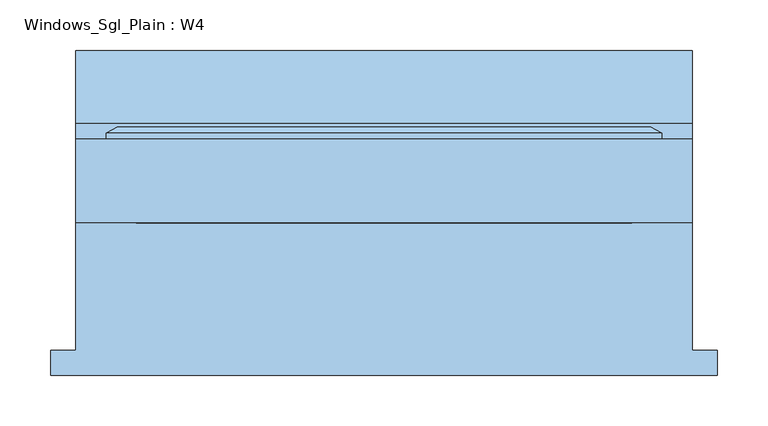
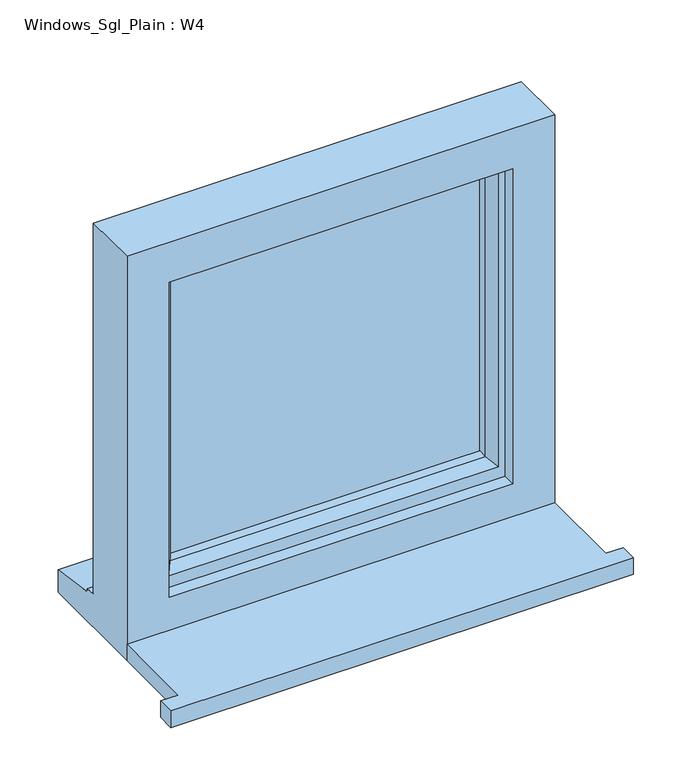
"""IFC4 building model written with IfcOpenShell, lengths in millimetres: window geometry, Windows_Sgl_Plain : W4."""

from ifc_helpers import new_model, si_unit, frame, origin, place, context, project, spatial, polyline, outline, extrude, faceted_brep, source, transform, mapped, element, save


def windows_sgl_plain_w4_5502dfe6(model_context):
    return source(origin(), model_context, "Body", "SolidModel", [
        extrude(outline(polyline([(-329.8, -146.0834322), (-329.8, -121.0834322), (-304.8, -121.0834322), (-304.8, 4.9965678), (304.8, 4.9965678), (304.8, -121.0834322), (329.8, -121.0834322), (329.8, -146.0834322), (-329.8, -146.0834322)])), frame((0.0, 0.0, 1500.4), z_axis=(0.0, 0.0, 1.0), x_axis=(1.0, 0.0, 0.0)), (0.0, 0.0, 1.0), 25.0),
        faceted_brep([(-304.8, 4.9965678, 1500.4), (304.8, 4.9965678, 1500.4), (304.8, 4.9965678, 2110.0), (-304.8, 4.9965678, 2110.0), (-244.8, 4.9965678, 2050.0), (244.8, 4.9965678, 2050.0), (244.8, 4.9965678, 1575.4), (-244.8, 4.9965678, 1575.4), (-304.8, 87.9965678, 2110.0), (-304.8, 87.9965678, 1551.4), (-304.8, 102.9965678, 1550.08767), (-304.8, 102.9965678, 1545.1449676), (-304.8, 175.4965678, 1534.2088847), (-304.8, 175.4965678, 1500.4), (304.8, 87.9965678, 2110.0), (304.8, 87.9965678, 1551.4), (-264.8, 87.9965678, 2070.0), (-264.8, 87.9965678, 1563.4), (264.8, 87.9965678, 1563.4), (264.8, 87.9965678, 2070.0), (-264.8, 22.9965678, 2070.0), (-264.8, 22.9965678, 1563.4), (264.8, 22.9965678, 2070.0), (264.8, 22.9965678, 1563.4), (-244.8, 22.9965678, 2050.0), (-244.8, 22.9965678, 1575.4), (244.8, 22.9965678, 1575.4), (244.8, 22.9965678, 2050.0), (304.8, 175.4965678, 1500.4), (304.8, 175.4965678, 1534.2088847), (304.8, 102.9965678, 1545.1449676), (304.8, 102.9965678, 1550.08767)], [[[0, 1, 2, 3], [4, 5, 6, 7]], [[0, 3, 8, 9, 10, 11, 12, 13]], [[9, 8, 14, 15], [16, 17, 18, 19]], [[17, 16, 20, 21]], [[20, 22, 23, 21], [24, 25, 26, 27]], [[24, 4, 7, 25]], [[3, 2, 14, 8]], [[16, 19, 22, 20]], [[5, 4, 24, 27]], [[15, 14, 2, 1, 28, 29, 30, 31]], [[19, 18, 23, 22]], [[5, 27, 26, 6]], [[28, 1, 0, 13]], [[29, 28, 13, 12]], [[30, 29, 12, 11]], [[31, 30, 11, 10]], [[15, 31, 10, 9]], [[21, 23, 18, 17]], [[7, 6, 26, 25]]]),
        extrude(outline(polyline([(234.8, 51.9965678), (-234.8, 51.9965678), (-234.8, 75.9965678), (234.8, 75.9965678), (234.8, 51.9965678)])), frame((0.0, 0.0, 1593.4), z_axis=(0.0, 0.0, 1.0), x_axis=(1.0, 0.0, 0.0)), (0.0, 0.0, 1.0), 446.6),
        faceted_brep([(-274.8, 87.9965678, 2080.0), (-274.8, 93.7700705, 2080.0), (-274.8, 93.7700705, 1553.4), (-274.8, 87.9965678, 1553.4), (-264.8, 22.9965678, 2070.0), (-264.8, 87.9965678, 2070.0), (-264.8, 87.9965678, 1563.4), (-264.8, 22.9965678, 1563.4), (-224.8, 37.4894677, 2030.0), (-234.9480377, 22.9965678, 2040.1480377), (-234.9480377, 22.9965678, 1593.2519623), (-224.8, 37.4894677, 1603.4), (-224.8, 51.9965678, 2030.0), (-224.8, 51.9965678, 1603.4), (-234.8, 75.9965678, 2040.0), (-234.8, 51.9965678, 2040.0), (-234.8, 51.9965678, 1593.4), (-234.8, 75.9965678, 1593.4), (-224.8, 93.7700705, 2030.0), (-224.8, 75.9965678, 2030.0), (-224.8, 75.9965678, 1603.4), (-224.8, 93.7700705, 1603.4), (-242.2457548, 99.5435732, 2047.4457548), (-242.2457548, 99.5435732, 1585.9542452), (-264.0153903, 99.5435732, 2069.2153903), (-264.0153903, 99.5435732, 1564.1846097), (274.8, 93.7700705, 1553.4), (274.8, 87.9965678, 1553.4), (264.8, 87.9965678, 1563.4), (264.8, 22.9965678, 1563.4), (234.9480377, 22.9965678, 1593.2519623), (224.8, 37.4894677, 1603.4), (224.8, 51.9965678, 1603.4), (234.8, 51.9965678, 1593.4), (234.8, 75.9965678, 1593.4), (224.8, 75.9965678, 1603.4), (224.8, 93.7700705, 1603.4), (242.2457548, 99.5435732, 1585.9542452), (264.0153903, 99.5435732, 1564.1846097), (274.8, 93.7700705, 2080.0), (274.8, 87.9965678, 2080.0), (264.8, 87.9965678, 2070.0), (264.8, 22.9965678, 2070.0), (234.9480377, 22.9965678, 2040.1480377), (224.8, 37.4894677, 2030.0), (224.8, 51.9965678, 2030.0), (234.8, 51.9965678, 2040.0), (234.8, 75.9965678, 2040.0), (224.8, 75.9965678, 2030.0), (224.8, 93.7700705, 2030.0), (242.2457548, 99.5435732, 2047.4457548), (264.0153903, 99.5435732, 2069.2153903)], [[[0, 1, 2, 3]], [[4, 5, 6, 7]], [[8, 9, 10, 11]], [[12, 8, 11, 13]], [[14, 15, 16, 17]], [[18, 19, 20, 21]], [[22, 18, 21, 23]], [[1, 24, 25, 2]], [[3, 2, 26, 27]], [[7, 6, 28, 29]], [[11, 10, 30, 31]], [[13, 11, 31, 32]], [[17, 16, 33, 34]], [[21, 20, 35, 36]], [[23, 21, 36, 37]], [[2, 25, 38, 26]], [[27, 26, 39, 40]], [[29, 28, 41, 42]], [[31, 30, 43, 44]], [[32, 31, 44, 45]], [[34, 33, 46, 47]], [[36, 35, 48, 49]], [[37, 36, 49, 50]], [[26, 38, 51, 39]], [[40, 39, 1, 0]], [[3, 27, 40, 0], [5, 41, 28, 6]], [[42, 41, 5, 4]], [[7, 29, 42, 4], [9, 43, 30, 10]], [[44, 43, 9, 8]], [[45, 44, 8, 12]], [[15, 46, 33, 16], [13, 32, 45, 12]], [[47, 46, 15, 14]], [[17, 34, 47, 14], [19, 48, 35, 20]], [[49, 48, 19, 18]], [[50, 49, 18, 22]], [[24, 51, 38, 25], [23, 37, 50, 22]], [[39, 51, 24, 1]]]),
    ])


if __name__ == "__main__":
    model = new_model("IFC4")
    model_context = context("Model", 3, world=origin())
    ifc_project = project(units=[si_unit("LENGTHUNIT", "METRE", prefix="MILLI")], contexts=[model_context])
    site = spatial("IfcSite", under=ifc_project)
    building = spatial("IfcBuilding", under=site)
    placement = place(None, origin())
    windows_sgl_plain_w4_shape = windows_sgl_plain_w4_5502dfe6(model_context)
    element("IfcWindow", 1, ObjectType="Windows_Sgl_Plain : W4", at=placement, inside=building, context=model_context, shape_type="MappedRepresentation", body=[
        mapped(windows_sgl_plain_w4_shape, transform((0.0, 0.0, 0.0), x_axis=(1.0, 0.0, 0.0), y_axis=(0.0, 1.0, 0.0), z_axis=(0.0, 0.0, 1.0))),
    ])
    save(model, "model.ifc")

# Revit data of these elements
# Type "Windows_Sgl_Plain : W4"
#   Type Mark = "59"
#   Operation = "SinglePanel"
#   Construction Type Id = "SGL"
#   Manufacturer = "Revit"
#   Keynote = "L10"
#   Analytic Construction = "Large single-glazed windows"
#   Wrap Layers (Ext) from Ext = 102.5 mm
#   Wrap Layers (Int) from Ext = 177.5 mm
#   Window Board Projection = 25 mm
#   Window Board Extension = 25 mm
#   Visual Light Transmittance = 0.9
#   Solar Heat Gain Coefficient = 0.86
#   Rough Width = 609.6 mm
#   Rough Height = 609.6 mm
#   Height = 609.6 mm
#   Width = 609.6 mm
#   Heat Transfer Coefficient (U) = 5.5617 W/(m²·K)
#   Glazing Thickness = 24 mm
#   FrameOffset - External = 50 mm
#   Frame Depth = 65 mm
#   Default Head Height = 2110 mm
#   Cill Depth = 87.5 mm
#   Cavity Closer Width = 50 mm
#   Cavity Closer Offset from Ext = 102.5 mm
#   Cavity Closer Depth = 85 mm
#   Vis - Cavity Closers = yes
#   Define Thermal Properties by = 1
#   Material Trim = Window Frame
#   Material Glass = Glass
#   Material Frame = Window Frame
#   Wall Closure = (empty or 0)
# Element 1 (IfcWindow, "Windows_Sgl_Plain : W4")
#   Materials on its faces: "Window Frame", "Glass"
# Materials
#   "Window Frame": colour RGB 249 249 249, transparency 0, Keynote = "L10", Cost = 0
#   "Glass": class "Glass", colour RGB 0 128 192, transparency 0.9, Description = "Soda Lime Glass", Cost = 0
